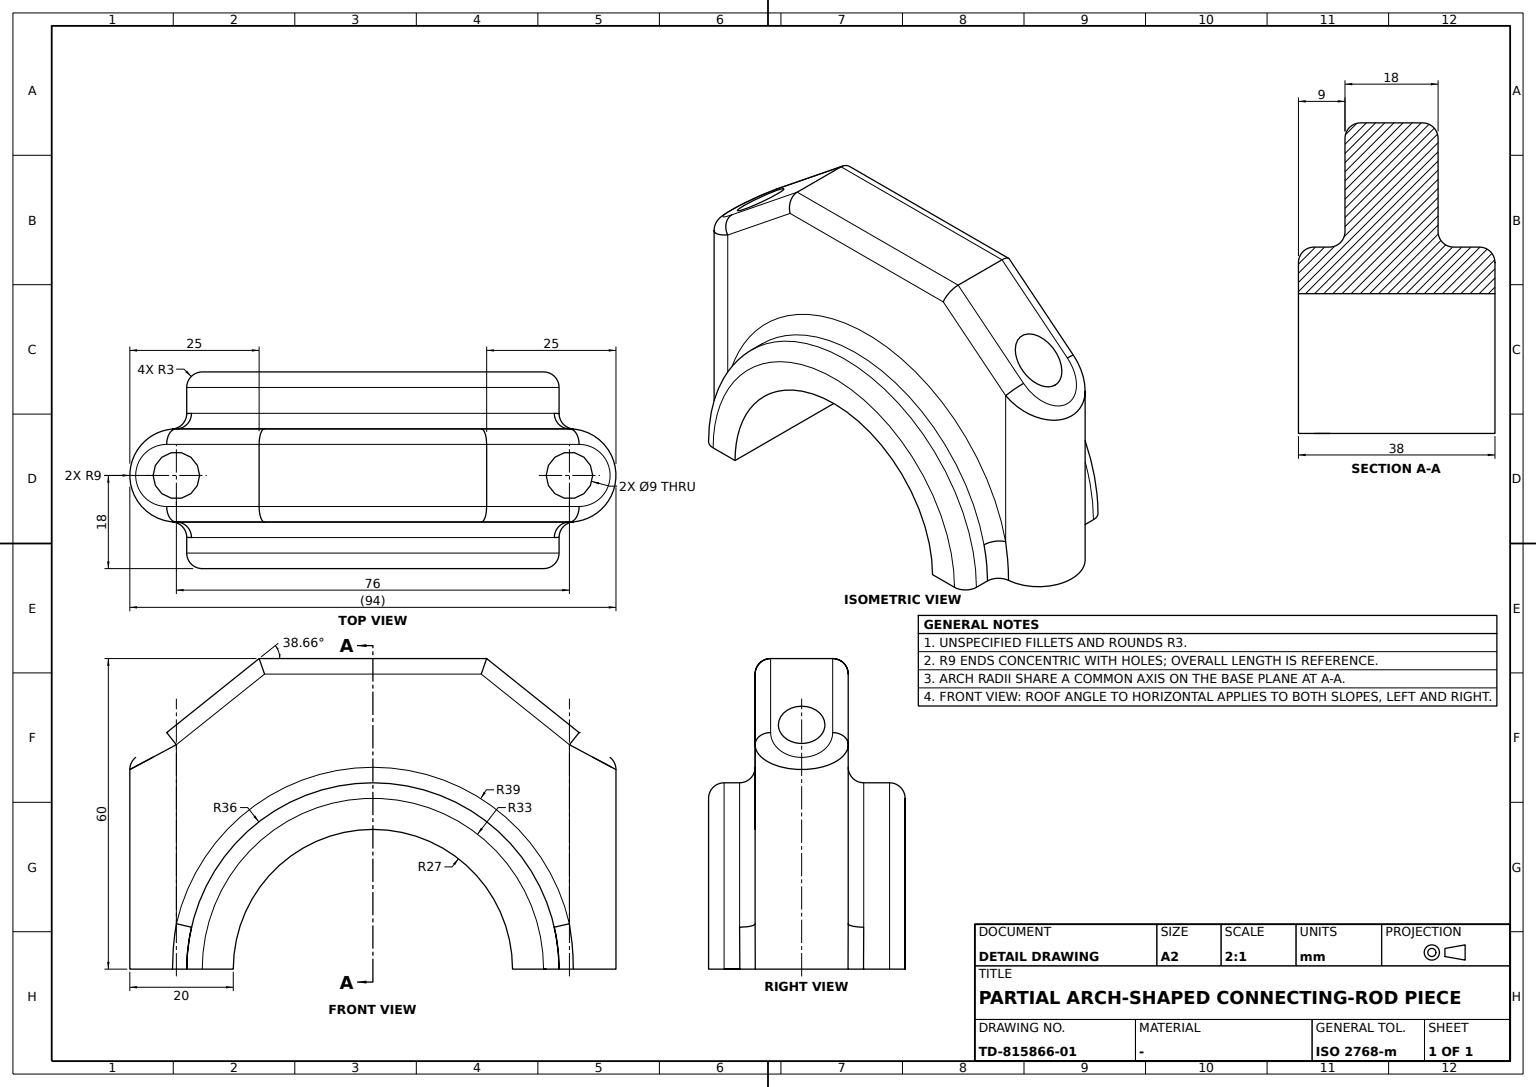
CATIA V5 part; units mm, degrees
sketch "Sketch1" plane through (0, 0, 0) normal (1, 0, 0) x (0, 1, 0)
  arc A0 (27, 0) -> (-27, 0) centre (0, 0) ccw
  arc A1 (36, 0) -> (-36, 0) centre (0, 0) ccw
  line L0 (-36, 0) -> (-27, 0)
  point P0 (-36, 0)
  point P1 (27, 0)
  line L1 (27, 0) -> (36, 0)
  dimension "radius A1" = 36
  dimension "radius A0" = 27
  constraint coincidence P0 x-axis
  constraint coincidence L0 P1
  constraint coincidence L0 L1
  constraint horizontal L0 x-axis
  constraint horizontal L1 x-axis
extrude "Pad1" add sketch "Sketch1" along normal blind 38
ref_plane "Plane1" through (0, 0, 60) normal (0, 0, 1) x (1, 0, 0)
sketch "Sketch2" plane through (0, 0, 60) normal (0, 0, 1) x (1, 0, 0)
  line L0 (20, 126.5252) -> (20, -50.5252) construction
  point P0 (20, 38)
  line L1 (11, -38) -> (11, 38)
  line L2 (29, 38) -> (29, -38)
  arc A0 (11, 38) -> (29, 38) centre (20, 38) cw
  arc A1 (29, -38) -> (11, -38) centre (20, -38) cw
  line L3 (0, 0) -> (38, 0) construction
  point P1 (38, 0)
  line L4 (38, 36) -> (38, -36) construction
  line L5 (20, 59.4748) -> (20, -40.5252) construction
  dimension "length L1" = 76
  dimension "distance L1 L5" = 9
  constraint vertical L0 y-axis
  constraint vertical L5 y-axis
  constraint midpoint P0 L0
  constraint tangency A0 L1
  constraint tangency A1 L1
  constraint tangency A0 L2
  constraint tangency A1 L2
  constraint horizontal L3 x-axis
  constraint coincidence P1 L4
  constraint symmetry L1 L2 L0
  constraint symmetry L2 L1 L5
  constraint symmetry A0 A1 L3
extrude "Pad2" add sketch "Sketch2" against normal up to surface (60 mm away)
sketch "Sketch3" plane through (29, 0, 0) normal (1, 0, 0) x (0, 1, 0)
  line L0 (-27, 0) -> (27, 0)
  arc A0 (27, 0) -> (-27, 0) centre (0, 0) ccw
  arc A1 (27, 0) -> (-27, 0) centre (0, 0) ccw construction
  constraint horizontal L0 x-axis
  constraint coincidence A1 A0
extrude "Pocket1" cut sketch "Sketch3" against normal blind 38
sketch "Sketch4" plane through (29, 0, 0) normal (1, 0, 0) x (0, 1, 0)
  point P0 (22, 60)
  line L0 (22, 60) -> (47, 60)
  point P1 (47, 60)
  line L1 (47, 60) -> (47, 40)
  point P2 (47, 40)
  line L2 (47, 40) -> (22, 60)
  line L3 (-38, 60) -> (38, 60) construction
  point P3 (-22, 60)
  point P4 (-47, 60)
  point P5 (-47, 40)
  line L4 (-22, 60) -> (-47, 60)
  line L5 (-47, 60) -> (-47, 40)
  line L6 (-47, 40) -> (-22, 60)
  dimension "distance L1 y axis" = 47
  dimension "length L1" = 20
  dimension "length L0" = 25
  constraint horizontal L0 x-axis
  constraint vertical L1 y-axis
  constraint coincidence L0 L3
  constraint symmetry P0 P3 y-axis
  constraint symmetry P1 P4 y-axis
  constraint symmetry P2 P5 y-axis
  constraint symmetry L0 L4 y-axis
  constraint symmetry L1 L5 y-axis
  constraint symmetry L2 L6 y-axis
extrude "Pocket2" cut sketch "Sketch4" against normal blind 38
sketch "Sketch6" plane through (0, 0, 0) normal (0, 0, -1) x (1, 0, 0)
  circle A0 centre (20, 38) radius 4.5
  arc A1 (29, 38) -> (11, 38) centre (20, 38) ccw construction
  circle A2 centre (20, -38) radius 4.5
  dimension "radius A0" = 4.5
  constraint concentricity A0 A1
  constraint symmetry A0 A2 x-axis
extrude "Pocket3" cut sketch "Sketch6" against normal through all
fillet "Fillet1" radius 3 8 edges at (29, 0, 36) (38, 0, 36) (29, 0, 60) (11, 0, 60) (29, -30, 53.6) (29, 30, 53.6) (11, 0, 36) (0, 0, 36)
sketch "Sketch5" plane through (0, 0, 0) normal (0, 0, -1) x (1, 0, 0)
